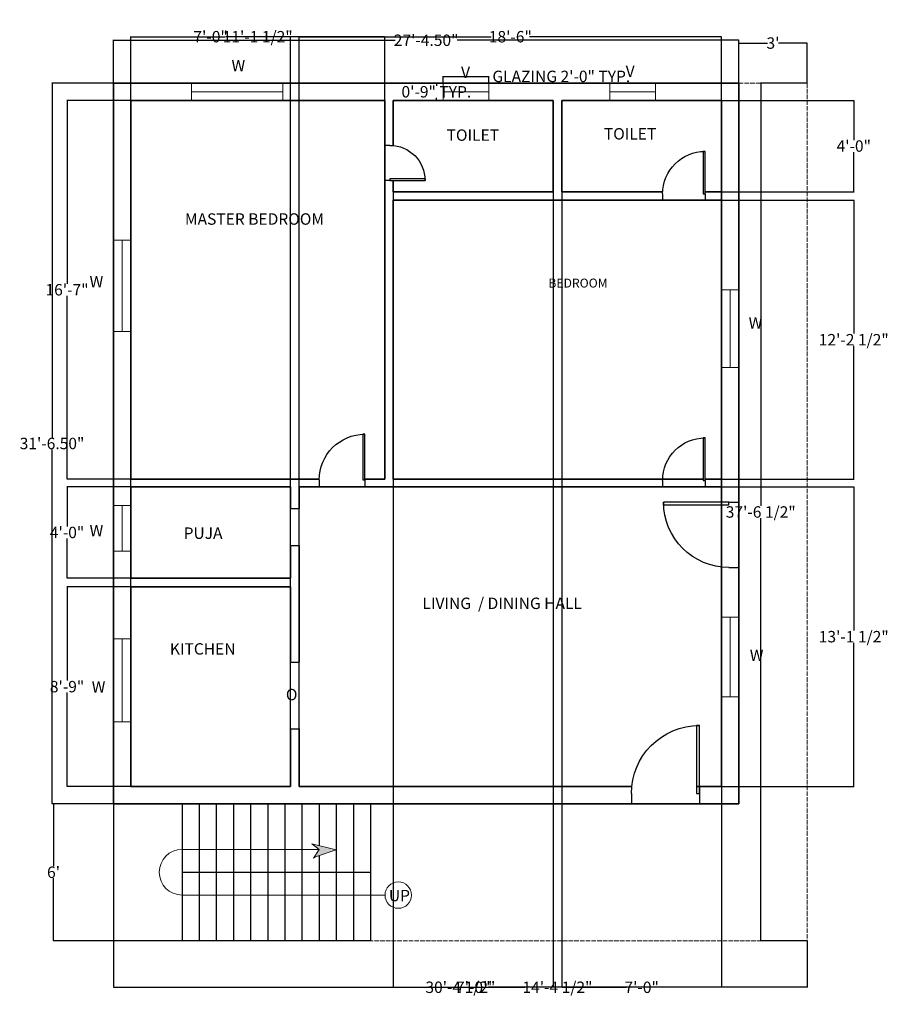
# Model space of a CAD drawing. Units: inches. Extents: x -21 to 896, y -151 to 366.
# Tile 2 of 2: x 440 to 896, y -151 to 366. Entities that reach past the tile are written whole.
import ezdxf

# ---------------------------------------------------------------- set-up
doc = ezdxf.new("R2010")
doc.units = ezdxf.units.IN
doc.header["$MEASUREMENT"] = 0
doc.linetypes.add('ACAD_ISO02W100', pattern=[15, 12, -3])
for name, color, linetype, lineweight in [('A-ANNO-DIMS', 2, 'Continuous', 18), ('A-ANNO-SYMB', 7, 'Continuous', 18), ('A-ANNO-TEXT', 7, 'Continuous', 18), ('A-AREA-IDEN', 7, 'Continuous', 25), ('A-DOOR', 3, 'Continuous', 25), ('A-FLOR-STRS', 7, 'Continuous', 25), ('A-GLAZ', 4, 'Continuous', 18), ('A-WALL', 7, 'Continuous', 35), ('A-WALL-OPEN', 7, 'ACAD_ISO02W100', 25), ('C-PROP', 8, 'ACAD_ISO02W100', 18)]:
    doc.layers.add(name, color=color, linetype=linetype, lineweight=lineweight)
doc.styles.get("Standard").update_dxf_attribs({"font": 'arial.ttf'})
doc.dimstyles.get("Standard").update_dxf_attribs({"dimtxt": 6, "dimasz": 0.18, "dimexe": 0.18, "dimexo": 0.0625, "dimgap": 0.09, "dimtad": 0, "dimtih": 1, "dimtoh": 1, "dimzin": 0, "dimdsep": 46, "dimlunit": 3, "dimtxsty": 'Standard', "dimcen": 0.09, "dimadec": 0, "dimazin": 0, "dimtfac": 1, "dimtofl": 0, "dimtmove": 0, "dimatfit": 3, "dimfxl": 1, "dimtolj": 1, "dimtzin": 0, "dimarcsym": 0})

# ---------------------------------------------------------------- blocks, each defined once
blk = doc.blocks.new('*U2')
for p, q in [((0, 0), (0, -6)), ((40, 0), (40, -6))]:
    blk.add_line(p, q)
blk.add_lwpolyline([(0, 0), (0, 40), (1.75, 40), (1.75, 0)], close=True)
blk.add_arc((0, 0), 40, 0, 90)
blk = doc.blocks.new('*D17')
at = {"layer": 'A-ANNO-DIMS', "color": 0, "lineweight": -2, "ltscale": 0.4, "transparency": 16777216}
for p, q in [((489.19, 332.75), (489.19, 355.46)), ((489.37, 355.28), (637.17, 355.28)), ((817.51, 355.28), (669.71, 355.28)), ((817.69, 332.75), (817.69, 355.46))]:
    blk.add_line(p, q, dxfattribs=at)
at = {"layer": 'A-ANNO-DIMS', "color": 0, "ltscale": 0.4, "transparency": 16777216}
for points in [[(489.37, 355.31), (489.37, 355.25), (489.19, 355.28)], [(817.51, 355.31), (817.51, 355.25), (817.69, 355.28)]]:
    blk.add_solid(points, dxfattribs=at)
at = {"layer": 'Defpoints', "color": 0, "ltscale": 0.4, "transparency": 16777216}
for p in [(817.69, 355.28), (489.19, 332.69), (817.69, 332.69)]:
    blk.add_point(p, dxfattribs=at)
at = {"layer": 'A-ANNO-DIMS', "color": 0, "ltscale": 0.4, "transparency": 16777216, "insert": (653.44, 355.28), "char_height": 6, "attachment_point": 5}
blk.add_mtext('\\A1;27\'-4.50"', dxfattribs=at)
blk = doc.blocks.new('*D18')
at = {"layer": 'A-ANNO-DIMS', "color": 0, "lineweight": -2, "ltscale": 0.4, "transparency": 16777216}
for p, q in [((489.13, 332.69), (456.69, 332.69)), ((456.87, 332.51), (456.87, 146.59)), ((456.87, -45.63), (456.87, 140.28)), ((489.13, -45.81), (456.69, -45.81))]:
    blk.add_line(p, q, dxfattribs=at)
at = {"layer": 'A-ANNO-DIMS', "color": 0, "ltscale": 0.4, "transparency": 16777216}
for points in [[(456.84, 332.51), (456.9, 332.51), (456.87, 332.69)], [(456.84, -45.63), (456.9, -45.63), (456.87, -45.81)]]:
    blk.add_solid(points, dxfattribs=at)
at = {"layer": 'Defpoints', "color": 0, "ltscale": 0.4, "transparency": 16777216}
for p in [(489.19, 332.69), (456.87, -45.81), (489.19, -45.81)]:
    blk.add_point(p, dxfattribs=at)
at = {"layer": 'A-ANNO-DIMS', "color": 0, "ltscale": 0.4, "transparency": 16777216, "insert": (456.87, 143.44), "char_height": 6, "attachment_point": 5}
blk.add_mtext('\\A1;31\'-6.50"', dxfattribs=at)
blk = doc.blocks.new('*D19')
at = {"layer": 'A-ANNO-DIMS', "color": 0, "lineweight": -2, "ltscale": 0.4, "transparency": 16777216}
for p, q in [((489.13, -45.81), (457.48, -45.81)), ((457.66, -45.99), (457.66, -78.66)), ((457.66, -117.63), (457.66, -84.97)), ((489.13, -117.81), (457.48, -117.81))]:
    blk.add_line(p, q, dxfattribs=at)
at = {"layer": 'A-ANNO-DIMS', "color": 0, "ltscale": 0.4, "transparency": 16777216}
for points in [[(457.63, -45.99), (457.69, -45.99), (457.66, -45.81)], [(457.63, -117.63), (457.69, -117.63), (457.66, -117.81)]]:
    blk.add_solid(points, dxfattribs=at)
at = {"layer": 'Defpoints', "color": 0, "ltscale": 0.4, "transparency": 16777216}
for p in [(489.19, -45.81), (457.66, -117.81), (489.19, -117.81)]:
    blk.add_point(p, dxfattribs=at)
at = {"layer": 'A-ANNO-DIMS', "color": 0, "ltscale": 0.4, "transparency": 16777216, "insert": (457.66, -81.81), "char_height": 6, "attachment_point": 5}
blk.add_mtext("\\A1;6'", dxfattribs=at)
blk = doc.blocks.new('*D20')
at = {"layer": 'A-ANNO-DIMS', "color": 0, "lineweight": -2, "ltscale": 0.4, "transparency": 16777216}
for p, q in [((817.69, 332.75), (817.69, 353.98)), ((817.87, 353.8), (832.84, 353.8)), ((853.51, 353.8), (838.54, 353.8)), ((853.69, 332.75), (853.69, 353.98))]:
    blk.add_line(p, q, dxfattribs=at)
at = {"layer": 'A-ANNO-DIMS', "color": 0, "ltscale": 0.4, "transparency": 16777216}
for points in [[(817.87, 353.83), (817.87, 353.77), (817.69, 353.8)], [(853.51, 353.83), (853.51, 353.77), (853.69, 353.8)]]:
    blk.add_solid(points, dxfattribs=at)
at = {"layer": 'Defpoints', "color": 0, "ltscale": 0.4, "transparency": 16777216}
for p in [(853.69, 353.8), (817.69, 332.69), (853.69, 332.69)]:
    blk.add_point(p, dxfattribs=at)
at = {"layer": 'A-ANNO-DIMS', "color": 0, "ltscale": 0.4, "transparency": 16777216, "insert": (835.69, 353.8), "char_height": 6, "attachment_point": 5}
blk.add_mtext("\\A1;3'", dxfattribs=at)
blk = doc.blocks.new('STAIR-RETURN-72IN')
for p, q in [((0, 72), (0, 0)), ((36, 72), (36, 0)), ((45, 72), (45, 0)), ((54, 72), (54, 0)), ((63, 72), (63, 0)), ((72, 72), (72, 0)), ((81, 72), (81, 0)), ((90, 72), (90, 0)), ((99, 72), (99, 0)), ((108, 72), (108, 50.05)), ((117, 72), (117, 0)), ((126, 72), (126, 0)), ((135, 72), (135, 0)), ((108, 44.67), (108, 0)), ((36, 36), (135, 36))]:
    blk.add_line(p, q)
blk.add_lwpolyline([(135, 0), (0, 0)])
blk = doc.blocks.new('STAIR-TRAVEL-UP')
h = blk.add_hatch(color=256)
h.dxf.hatch_style = 1
h.paths.add_polyline_path([(-32.62, 23.79), (-45.42, 26.99), (-41.62, 24), (-44.5, 19.46), (-43.01, 20.19)])
for p, q in [((-41.62, 24), (-45.42, 26.99)), ((-45.42, 26.99), (-32.62, 23.79)), ((-113.62, 24), (-41.62, 24)), ((-44.5, 19.46), (-41.62, 24)), ((-32.62, 23.79), (-43.01, 20.19)), ((-43.01, 20.19), (-44.5, 19.46)), ((-113.62, 0), (-14.62, 0)), ((-14.62, 0), (-6.96, 0))]:
    blk.add_line(p, q)
blk.add_circle((0, 0), 6.96)
blk.add_arc((-113.62, 12), 12, 90, 270)
at = {"insert": (-4.95, 2.74), "char_height": 6, "attachment_point": 1}
blk.add_mtext_dynamic_manual_height_columns('UP', width=3.031, gutter_width=1, heights=[0.203], dxfattribs=at)
blk = doc.blocks.new('WIN-48IN')
at = {"ltscale": 0.4}
for p, q in [((0, 9), (0, 0)), ((48, 9), (48, 0)), ((0, 4.5), (48, 4.5))]:
    blk.add_line(p, q, dxfattribs=at)
blk = doc.blocks.new('GLAZ-24IN')
at = {"ltscale": 0.4}
for p, q in [((0, 9), (0, 0)), ((24, 9), (24, 0)), ((0, 4.5), (24, 4.5))]:
    blk.add_line(p, q, dxfattribs=at)
blk = doc.blocks.new('*D27')
at = {"layer": 'A-ANNO-DIMS', "color": 0, "lineweight": -2, "ltscale": 0.4, "transparency": 16777216}
for p, q in [((662.4, 332.75), (662.4, 336.47)), ((662.58, 336.29), (686.22, 336.29)), ((686.4, 332.75), (686.4, 336.47)), ((686.4, 336.29), (686.58, 336.29))]:
    blk.add_line(p, q, dxfattribs=at)
at = {"layer": 'A-ANNO-DIMS', "color": 0, "ltscale": 0.4, "transparency": 16777216}
for points in [[(662.58, 336.32), (662.58, 336.26), (662.4, 336.29)], [(686.22, 336.32), (686.22, 336.26), (686.4, 336.29)]]:
    blk.add_solid(points, dxfattribs=at)
at = {"layer": 'Defpoints', "color": 0, "ltscale": 0.4, "transparency": 16777216}
for p in [(686.4, 336.29), (662.4, 332.69), (686.4, 332.69)]:
    blk.add_point(p, dxfattribs=at)
at = {"layer": 'A-ANNO-DIMS', "color": 0, "ltscale": 0.4, "transparency": 16777216, "insert": (724.47, 336.29), "char_height": 6, "attachment_point": 5}
blk.add_mtext('\\A1;GLAZING 2\'-0" TYP.', dxfattribs=at)
blk = doc.blocks.new('*D28')
at = {"layer": 'A-ANNO-DIMS', "color": 0, "lineweight": -2, "ltscale": 0.4, "transparency": 16777216}
for p, q in [((662.33, 332.69), (658.62, 332.69)), ((658.8, 332.51), (658.8, 331.34)), ((662.33, 323.69), (658.62, 323.69)), ((658.8, 323.87), (658.8, 325.03))]:
    blk.add_line(p, q, dxfattribs=at)
at = {"layer": 'A-ANNO-DIMS', "color": 0, "ltscale": 0.4, "transparency": 16777216}
for points in [[(658.77, 332.51), (658.83, 332.51), (658.8, 332.69)], [(658.77, 323.87), (658.83, 323.87), (658.8, 323.69)]]:
    blk.add_solid(points, dxfattribs=at)
at = {"layer": 'Defpoints', "color": 0, "ltscale": 0.4, "transparency": 16777216}
for p in [(658.8, 332.69), (662.4, 332.69), (662.4, 323.69)]:
    blk.add_point(p, dxfattribs=at)
at = {"layer": 'A-ANNO-DIMS', "color": 0, "ltscale": 0.4, "transparency": 16777216, "insert": (658.8, 328.19), "char_height": 6, "attachment_point": 5}
blk.add_mtext('\\A1;0\'-9" TYP.', dxfattribs=at)
blk = doc.blocks.new('*D33')
at = {"layer": 'A-ANNO-DIMS', "color": 0, "lineweight": -2, "ltscale": 0.4, "transparency": 16777216}
for p, q in [((498.19, 323.75), (498.19, 357.31)), ((498.37, 357.13), (547.84, 357.13)), ((631.51, 357.13), (582.04, 357.13)), ((631.69, 323.75), (631.69, 357.31))]:
    blk.add_line(p, q, dxfattribs=at)
at = {"layer": 'A-ANNO-DIMS', "color": 0, "ltscale": 0.4, "transparency": 16777216}
for points in [[(498.37, 357.16), (498.37, 357.1), (498.19, 357.13)], [(631.51, 357.16), (631.51, 357.1), (631.69, 357.13)]]:
    blk.add_solid(points, dxfattribs=at)
at = {"layer": 'Defpoints', "color": 0, "ltscale": 0.4, "transparency": 16777216}
for p in [(631.69, 357.13), (498.19, 323.69), (631.69, 323.69)]:
    blk.add_point(p, dxfattribs=at)
at = {"layer": 'A-ANNO-DIMS', "color": 0, "ltscale": 0.4, "transparency": 16777216, "insert": (564.94, 357.13), "char_height": 6, "attachment_point": 5}
blk.add_mtext('\\A1;11\'-1 1/2"', dxfattribs=at)
blk = doc.blocks.new('*D34')
at = {"layer": 'A-ANNO-DIMS', "color": 0, "lineweight": -2, "ltscale": 0.4, "transparency": 16777216}
for p, q in [((498.13, 323.69), (464.57, 323.69)), ((464.75, 323.51), (464.75, 227.34)), ((464.75, 124.87), (464.75, 221.03)), ((498.13, 124.69), (464.57, 124.69))]:
    blk.add_line(p, q, dxfattribs=at)
at = {"layer": 'A-ANNO-DIMS', "color": 0, "ltscale": 0.4, "transparency": 16777216}
for points in [[(464.72, 323.51), (464.78, 323.51), (464.75, 323.69)], [(464.72, 124.87), (464.78, 124.87), (464.75, 124.69)]]:
    blk.add_solid(points, dxfattribs=at)
at = {"layer": 'Defpoints', "color": 0, "ltscale": 0.4, "transparency": 16777216}
for p in [(464.75, 323.69), (498.19, 323.69), (498.19, 124.69)]:
    blk.add_point(p, dxfattribs=at)
at = {"layer": 'A-ANNO-DIMS', "color": 0, "ltscale": 0.4, "transparency": 16777216, "insert": (464.75, 224.19), "char_height": 6, "attachment_point": 5}
blk.add_mtext('\\A1;16\'-7"', dxfattribs=at)
blk = doc.blocks.new('*D35')
at = {"layer": 'A-ANNO-DIMS', "color": 0, "lineweight": -2, "ltscale": 0.4, "transparency": 16777216}
for p, q in [((636.19, 124.62), (636.19, -142.43)), ((808.69, 124.62), (808.69, -142.43)), ((636.37, -142.25), (705.34, -142.25)), ((808.51, -142.25), (739.54, -142.25))]:
    blk.add_line(p, q, dxfattribs=at)
at = {"layer": 'A-ANNO-DIMS', "color": 0, "ltscale": 0.4, "transparency": 16777216}
for points in [[(636.37, -142.22), (636.37, -142.28), (636.19, -142.25)], [(808.51, -142.22), (808.51, -142.28), (808.69, -142.25)]]:
    blk.add_solid(points, dxfattribs=at)
at = {"layer": 'Defpoints', "color": 0, "ltscale": 0.4, "transparency": 16777216}
for p in [(636.19, 124.69), (808.69, 124.69), (808.69, -142.25)]:
    blk.add_point(p, dxfattribs=at)
at = {"layer": 'A-ANNO-DIMS', "color": 0, "ltscale": 0.4, "transparency": 16777216, "insert": (722.44, -142.25), "char_height": 6, "attachment_point": 5}
blk.add_mtext('\\A1;14\'-4 1/2"', dxfattribs=at)
blk = doc.blocks.new('*D36')
at = {"layer": 'A-ANNO-DIMS', "color": 0, "lineweight": -2, "ltscale": 0.4, "transparency": 16777216}
for p, q in [((636.19, 275.62), (636.19, -142.43)), ((720.19, 275.62), (720.19, -142.43)), ((636.37, -142.25), (670.15, -142.25)), ((720.01, -142.25), (686.23, -142.25))]:
    blk.add_line(p, q, dxfattribs=at)
at = {"layer": 'A-ANNO-DIMS', "color": 0, "ltscale": 0.4, "transparency": 16777216}
for points in [[(636.37, -142.22), (636.37, -142.28), (636.19, -142.25)], [(720.01, -142.22), (720.01, -142.28), (720.19, -142.25)]]:
    blk.add_solid(points, dxfattribs=at)
at = {"layer": 'Defpoints', "color": 0, "ltscale": 0.4, "transparency": 16777216}
for p in [(636.19, 275.69), (720.19, 275.69), (720.19, -142.25)]:
    blk.add_point(p, dxfattribs=at)
at = {"layer": 'A-ANNO-DIMS', "color": 0, "ltscale": 0.4, "transparency": 16777216, "insert": (678.19, -142.25), "char_height": 6, "attachment_point": 5}
blk.add_mtext('\\A1;7\'-0"', dxfattribs=at)
blk = doc.blocks.new('*D37')
at = {"layer": 'A-ANNO-DIMS', "color": 0, "lineweight": -2, "ltscale": 0.4, "transparency": 16777216}
for p, q in [((724.69, 275.62), (724.69, -142.43)), ((808.69, 275.62), (808.69, -142.43)), ((724.87, -142.25), (758.65, -142.25)), ((808.51, -142.25), (774.73, -142.25))]:
    blk.add_line(p, q, dxfattribs=at)
at = {"layer": 'A-ANNO-DIMS', "color": 0, "ltscale": 0.4, "transparency": 16777216}
for points in [[(724.87, -142.22), (724.87, -142.28), (724.69, -142.25)], [(808.51, -142.22), (808.51, -142.28), (808.69, -142.25)]]:
    blk.add_solid(points, dxfattribs=at)
at = {"layer": 'Defpoints', "color": 0, "ltscale": 0.4, "transparency": 16777216}
for p in [(724.69, 275.69), (808.69, 275.69), (808.69, -142.25)]:
    blk.add_point(p, dxfattribs=at)
at = {"layer": 'A-ANNO-DIMS', "color": 0, "ltscale": 0.4, "transparency": 16777216, "insert": (766.69, -142.25), "char_height": 6, "attachment_point": 5}
blk.add_mtext('\\A1;7\'-0"', dxfattribs=at)
blk = doc.blocks.new('*D38')
at = {"layer": 'A-ANNO-DIMS', "color": 0, "lineweight": -2, "ltscale": 0.4, "transparency": 16777216}
for p, q in [((808.75, 323.69), (878.31, 323.69)), ((878.13, 323.51), (878.13, 302.84)), ((878.13, 275.87), (878.13, 296.53)), ((808.75, 275.69), (878.31, 275.69))]:
    blk.add_line(p, q, dxfattribs=at)
at = {"layer": 'A-ANNO-DIMS', "color": 0, "ltscale": 0.4, "transparency": 16777216}
for points in [[(878.1, 323.51), (878.16, 323.51), (878.13, 323.69)], [(878.1, 275.87), (878.16, 275.87), (878.13, 275.69)]]:
    blk.add_solid(points, dxfattribs=at)
at = {"layer": 'Defpoints', "color": 0, "ltscale": 0.4, "transparency": 16777216}
for p in [(808.69, 323.69), (878.13, 323.69), (808.69, 275.69)]:
    blk.add_point(p, dxfattribs=at)
at = {"layer": 'A-ANNO-DIMS', "color": 0, "ltscale": 0.4, "transparency": 16777216, "insert": (878.13, 299.69), "char_height": 6, "attachment_point": 5}
blk.add_mtext('\\A1;4\'-0"', dxfattribs=at)
blk = doc.blocks.new('*D39')
at = {"layer": 'A-ANNO-DIMS', "color": 0, "lineweight": -2, "ltscale": 0.4, "transparency": 16777216}
for p, q in [((808.75, 271.19), (878.31, 271.19)), ((878.13, 271.01), (878.13, 201.13)), ((878.13, 124.87), (878.13, 194.74)), ((808.75, 124.69), (878.31, 124.69))]:
    blk.add_line(p, q, dxfattribs=at)
at = {"layer": 'A-ANNO-DIMS', "color": 0, "ltscale": 0.4, "transparency": 16777216}
for points in [[(878.1, 271.01), (878.16, 271.01), (878.13, 271.19)], [(878.1, 124.87), (878.16, 124.87), (878.13, 124.69)]]:
    blk.add_solid(points, dxfattribs=at)
at = {"layer": 'Defpoints', "color": 0, "ltscale": 0.4, "transparency": 16777216}
for p in [(808.69, 271.19), (878.13, 271.19), (808.69, 124.69)]:
    blk.add_point(p, dxfattribs=at)
at = {"layer": 'A-ANNO-DIMS', "color": 0, "ltscale": 0.4, "transparency": 16777216, "insert": (878.13, 197.94), "char_height": 6, "attachment_point": 5}
blk.add_mtext('\\A1;12\'-2 1/2"', dxfattribs=at)
blk = doc.blocks.new('*D40')
at = {"layer": 'A-ANNO-DIMS', "color": 0, "lineweight": -2, "ltscale": 0.4, "transparency": 16777216}
for p, q in [((808.75, 120.69), (878.31, 120.69)), ((878.13, 120.51), (878.13, 45.13)), ((878.13, -36.63), (878.13, 38.74)), ((808.75, -36.81), (878.31, -36.81))]:
    blk.add_line(p, q, dxfattribs=at)
at = {"layer": 'A-ANNO-DIMS', "color": 0, "ltscale": 0.4, "transparency": 16777216}
for points in [[(878.1, 120.51), (878.16, 120.51), (878.13, 120.69)], [(878.1, -36.63), (878.16, -36.63), (878.13, -36.81)]]:
    blk.add_solid(points, dxfattribs=at)
at = {"layer": 'Defpoints', "color": 0, "ltscale": 0.4, "transparency": 16777216}
for p in [(808.69, 120.69), (878.13, 120.69), (808.69, -36.81)]:
    blk.add_point(p, dxfattribs=at)
at = {"layer": 'A-ANNO-DIMS', "color": 0, "ltscale": 0.4, "transparency": 16777216, "insert": (878.13, 41.94), "char_height": 6, "attachment_point": 5}
blk.add_mtext('\\A1;13\'-1 1/2"', dxfattribs=at)
blk = doc.blocks.new('*D41')
at = {"layer": 'A-ANNO-DIMS', "color": 0, "lineweight": -2, "ltscale": 0.4, "transparency": 16777216}
for p, q in [((498.19, -36.75), (498.19, 357.31)), ((498.37, 357.13), (532.15, 357.13)), ((582.01, 357.13), (548.23, 357.13)), ((582.19, -36.75), (582.19, 357.31))]:
    blk.add_line(p, q, dxfattribs=at)
at = {"layer": 'A-ANNO-DIMS', "color": 0, "ltscale": 0.4, "transparency": 16777216}
for points in [[(498.37, 357.16), (498.37, 357.1), (498.19, 357.13)], [(582.01, 357.16), (582.01, 357.1), (582.19, 357.13)]]:
    blk.add_solid(points, dxfattribs=at)
at = {"layer": 'Defpoints', "color": 0, "ltscale": 0.4, "transparency": 16777216}
for p in [(582.19, 357.13), (498.19, -36.81), (582.19, -36.81)]:
    blk.add_point(p, dxfattribs=at)
at = {"layer": 'A-ANNO-DIMS', "color": 0, "ltscale": 0.4, "transparency": 16777216, "insert": (540.19, 357.13), "char_height": 6, "attachment_point": 5}
blk.add_mtext('\\A1;7\'-0"', dxfattribs=at)
blk = doc.blocks.new('*D42')
at = {"layer": 'A-ANNO-DIMS', "color": 0, "lineweight": -2, "ltscale": 0.4, "transparency": 16777216}
for p, q in [((586.69, -36.75), (586.69, 357.31)), ((586.87, 357.13), (687.58, 357.13)), ((808.51, 357.13), (707.8, 357.13)), ((808.69, -36.75), (808.69, 357.31))]:
    blk.add_line(p, q, dxfattribs=at)
at = {"layer": 'A-ANNO-DIMS', "color": 0, "ltscale": 0.4, "transparency": 16777216}
for points in [[(586.87, 357.16), (586.87, 357.1), (586.69, 357.13)], [(808.51, 357.16), (808.51, 357.1), (808.69, 357.13)]]:
    blk.add_solid(points, dxfattribs=at)
at = {"layer": 'Defpoints', "color": 0, "ltscale": 0.4, "transparency": 16777216}
for p in [(808.69, 357.13), (586.69, -36.81), (808.69, -36.81)]:
    blk.add_point(p, dxfattribs=at)
at = {"layer": 'A-ANNO-DIMS', "color": 0, "ltscale": 0.4, "transparency": 16777216, "insert": (697.69, 357.13), "char_height": 6, "attachment_point": 5}
blk.add_mtext('\\A1;18\'-6"', dxfattribs=at)
blk = doc.blocks.new('*D43')
at = {"layer": 'A-ANNO-DIMS', "color": 0, "lineweight": -2, "ltscale": 0.4, "transparency": 16777216}
for p, q in [((498.13, 68.19), (464.57, 68.19)), ((464.75, 68.01), (464.75, 18.84)), ((464.75, -36.63), (464.75, 12.53)), ((498.13, -36.81), (464.57, -36.81))]:
    blk.add_line(p, q, dxfattribs=at)
at = {"layer": 'A-ANNO-DIMS', "color": 0, "ltscale": 0.4, "transparency": 16777216}
for points in [[(464.72, 68.01), (464.78, 68.01), (464.75, 68.19)], [(464.72, -36.63), (464.78, -36.63), (464.75, -36.81)]]:
    blk.add_solid(points, dxfattribs=at)
at = {"layer": 'Defpoints', "color": 0, "ltscale": 0.4, "transparency": 16777216}
for p in [(464.75, 68.19), (498.19, 68.19), (498.19, -36.81)]:
    blk.add_point(p, dxfattribs=at)
at = {"layer": 'A-ANNO-DIMS', "color": 0, "ltscale": 0.4, "transparency": 16777216, "insert": (464.75, 15.69), "char_height": 6, "attachment_point": 5}
blk.add_mtext('\\A1;8\'-9"', dxfattribs=at)
blk = doc.blocks.new('*D44')
at = {"layer": 'A-ANNO-DIMS', "color": 0, "lineweight": -2, "ltscale": 0.4, "transparency": 16777216}
for p, q in [((498.13, 120.69), (464.57, 120.69)), ((464.75, 120.51), (464.75, 99.84)), ((464.75, 72.87), (464.75, 93.53)), ((498.13, 72.69), (464.57, 72.69))]:
    blk.add_line(p, q, dxfattribs=at)
at = {"layer": 'A-ANNO-DIMS', "color": 0, "ltscale": 0.4, "transparency": 16777216}
for points in [[(464.72, 120.51), (464.78, 120.51), (464.75, 120.69)], [(464.72, 72.87), (464.78, 72.87), (464.75, 72.69)]]:
    blk.add_solid(points, dxfattribs=at)
at = {"layer": 'Defpoints', "color": 0, "ltscale": 0.4, "transparency": 16777216}
for p in [(464.75, 120.69), (498.19, 120.69), (498.19, 72.69)]:
    blk.add_point(p, dxfattribs=at)
at = {"layer": 'A-ANNO-DIMS', "color": 0, "ltscale": 0.4, "transparency": 16777216, "insert": (464.75, 96.69), "char_height": 6, "attachment_point": 5}
blk.add_mtext('\\A1;4\'-0"', dxfattribs=at)
blk = doc.blocks.new('*D45')
at = {"layer": 'A-ANNO-DIMS', "color": 0, "lineweight": -2, "ltscale": 0.4, "transparency": 16777216}
for p, q in [((853.63, 332.69), (829.07, 332.69)), ((829.25, 332.51), (829.25, 110.63)), ((829.25, -117.63), (829.25, 104.24)), ((853.63, -117.81), (829.07, -117.81))]:
    blk.add_line(p, q, dxfattribs=at)
at = {"layer": 'A-ANNO-DIMS', "color": 0, "ltscale": 0.4, "transparency": 16777216}
for points in [[(829.22, 332.51), (829.28, 332.51), (829.25, 332.69)], [(829.22, -117.63), (829.28, -117.63), (829.25, -117.81)]]:
    blk.add_solid(points, dxfattribs=at)
at = {"layer": 'Defpoints', "color": 0, "ltscale": 0.4, "transparency": 16777216}
for p in [(829.25, 332.69), (853.69, 332.69), (853.69, -117.81)]:
    blk.add_point(p, dxfattribs=at)
at = {"layer": 'A-ANNO-DIMS', "color": 0, "ltscale": 0.4, "transparency": 16777216, "insert": (829.25, 107.44), "char_height": 6, "attachment_point": 5}
blk.add_mtext('\\A1;37\'-6 1/2"', dxfattribs=at)
blk = doc.blocks.new('*D46')
at = {"layer": 'A-ANNO-DIMS', "color": 0, "lineweight": -2, "ltscale": 0.4, "transparency": 16777216}
for p, q in [((489.19, -117.88), (489.19, -142.43)), ((853.69, -117.88), (853.69, -142.43)), ((489.37, -142.25), (654.05, -142.25)), ((853.51, -142.25), (688.82, -142.25))]:
    blk.add_line(p, q, dxfattribs=at)
at = {"layer": 'A-ANNO-DIMS', "color": 0, "ltscale": 0.4, "transparency": 16777216}
for points in [[(489.37, -142.22), (489.37, -142.28), (489.19, -142.25)], [(853.51, -142.22), (853.51, -142.28), (853.69, -142.25)]]:
    blk.add_solid(points, dxfattribs=at)
at = {"layer": 'Defpoints', "color": 0, "ltscale": 0.4, "transparency": 16777216}
for p in [(489.19, -117.81), (853.69, -117.81), (853.69, -142.25)]:
    blk.add_point(p, dxfattribs=at)
at = {"layer": 'A-ANNO-DIMS', "color": 0, "ltscale": 0.4, "transparency": 16777216, "insert": (671.44, -142.25), "char_height": 6, "attachment_point": 5}
blk.add_mtext('\\A1;30\'-4 1/2"', dxfattribs=at)

msp = doc.modelspace()

# ---------------------------------------------------------------- linework, layer by layer
at = {"layer": 'A-DOOR'}
msp.add_line((797.01, -36.815), (797.01, -45.815), dxfattribs=at)
at = {"layer": 'A-GLAZ', "ltscale": 0.4}
for p, q in [((749.973, 323.685), (749.973, 332.685)), ((773.973, 323.685), (773.973, 332.685)), ((749.973, 328.145), (773.973, 328.185)), ((808.689, 224.185), (817.689, 224.185)), ((813.189, 183.392), (813.189, 224.185)), ((808.689, 183.392), (817.689, 183.392)), ((808.689, 52.137), (817.689, 52.137)), ((813.189, 10.257), (813.189, 52.137)), ((489.189, 40.836), (498.189, 40.836)), ((493.689, -2.772), (493.689, 40.836)), ((808.689, 10.257), (817.689, 10.257)), ((489.189, -2.772), (498.189, -2.772))]:
    msp.add_line(p, q, dxfattribs=at)
at = {"layer": 'A-WALL'}
msp.add_lwpolyline([(489.189, 332.685), (817.689, 332.685), (817.689, -45.815), (489.189, -45.815)], close=True, dxfattribs=at)
for points in [[(498.189, 323.685), (631.689, 323.685)], [(498.189, 124.685), (498.189, 323.685)], [(631.689, 124.685), (631.689, 323.685)], [(636.189, 323.685), (636.189, 299.953)], [(636.189, 323.685), (720.189, 323.685)], [(720.189, 323.685), (720.189, 275.685)], [(724.689, 323.685), (724.689, 275.685)], [(724.689, 323.685), (808.689, 323.685)], [(808.689, 323.685), (808.689, 124.685)], [(636.189, 281.612), (636.189, 275.685)], [(636.189, 275.685), (720.189, 275.685)], [(724.689, 275.685), (777.724, 275.685)], [(800.066, 275.685), (808.689, 275.685)], [(636.189, 271.185), (808.689, 271.185)], [(636.189, 271.185), (636.189, 124.685)], [(724.689, 271.185), (808.689, 271.185)], [(498.189, 124.685), (597.248, 124.685)], [(621.257, 124.685), (631.689, 124.685)], [(636.189, 124.685), (799.087, 124.685)], [(800.066, 124.685), (808.689, 124.685)], [(498.189, 120.685), (582.189, 120.685)], [(498.189, 72.685), (498.189, 120.685)], [(582.189, 109.238), (582.189, 120.685)], [(586.689, 120.685), (808.689, 120.685)], [(586.689, 109.238), (586.689, 120.685)], [(808.689, 120.685), (808.689, 112.622)], [(582.189, 72.685), (582.189, 89.787)], [(586.689, 28.488), (586.689, 89.787)], [(808.689, 78.478), (808.689, -36.815)], [(498.189, 72.685), (582.189, 72.685)], [(498.189, -36.815), (498.189, 68.185)], [(498.189, 68.185), (582.189, 68.185)], [(582.189, 28.488), (582.189, 68.185)], [(582.189, -36.815), (582.189, -6.471)], [(586.689, -36.815), (586.689, -6.471)], [(582.189, -36.815), (498.189, -36.815)], [(761.466, -36.815), (586.689, -36.815)], [(808.689, -36.815), (795.447, -36.815)]]:
    msp.add_lwpolyline(points, dxfattribs=at)
at = {"layer": 'A-WALL-OPEN', "ltscale": 0.4}
for p, q in [((582.189, 109.238), (586.689, 109.238)), ((582.189, 89.787), (586.689, 89.787)), ((582.189, 28.488), (586.689, 28.488)), ((582.189, -6.471), (586.689, -6.471))]:
    msp.add_line(p, q, dxfattribs=at)
at = {"layer": 'C-PROP', "ltscale": 0.2}
msp.add_line((817.689, 332.685), (853.689, 332.685), dxfattribs=at)
for points in [[(853.689, 332.685), (853.689, -117.815)], [(853.689, -117.815), (624.189, -117.815)]]:
    msp.add_lwpolyline(points, dxfattribs=at)

# ---------------------------------------------------------------- block references
at = {"layer": 'A-ANNO-SYMB'}
msp.add_blockref('STAIR-TRAVEL-UP', (638.811, -93.815), dxfattribs=at)
at = {"layer": 'A-DOOR'}
for p, xscale, yscale, zscale, rotation in [((634.429, 281.612), -0.4606261510920194, 0.4606261510920194, 0.4606261510920194, 270), ((812.535, 112.622), -0.8590067270063272, 0.8590067270063272, 0.8590067270063272, 90)]:
    msp.add_blockref('*U2', p, dxfattribs=dict(at, xscale=xscale, yscale=yscale, zscale=zscale, rotation=rotation))
for p, xscale, yscale, zscale in [((800.066, 274.541), -0.5592774159886474, 0.5592774159886474, 0.5592774159886474), ((621.257, 124.287), -0.6002384071363702, 0.6002384071363702, 0.6002384071363702), ((800.066, 124.041), -0.5592774159886474, 0.5592774159886474, 0.5592774159886474), ((797.01, -40.455), -0.8932506770278118, 0.8932506770278118, 0.8932506770278118)]:
    msp.add_blockref('*U2', p, dxfattribs=dict(at, xscale=xscale, yscale=yscale, zscale=zscale))
at = {"layer": 'A-FLOR-STRS'}
msp.add_blockref('STAIR-RETURN-72IN', (489.189, -117.815), dxfattribs=at)
at = {"layer": 'A-GLAZ'}
for name, p in [('WIN-48IN', (530.078, 323.685)), ('GLAZ-24IN', (662.396, 323.685))]:
    msp.add_blockref(name, p, dxfattribs=at)
at = {"layer": 'A-GLAZ', "rotation": 270}
for name, p in [('WIN-48IN', (489.189, 250.261)), ('GLAZ-24IN', (489.189, 110.854))]:
    msp.add_blockref(name, p, dxfattribs=at)

# ---------------------------------------------------------------- texts
at = {"layer": 'A-ANNO-TEXT', "char_height": 6, "attachment_point": 1}
for s, insert in [('W', (551.178, 344.962)), ('V', (671.786, 341.404)), ('V', (758.297, 341.993)), ('W', (476.601, 231.392)), ('W', (822.897, 209.769)), ('W', (476.601, 100.668)), ('W', (823.509, 35.165)), ('W', (477.72, 18.546)), ('O', (579.745, 14.495))]:
    msp.add_mtext_dynamic_manual_height_columns(s, width=6, gutter_width=1, heights=[0.203], dxfattribs=dict(at, insert=insert))
at = {"layer": 'A-AREA-IDEN', "attachment_point": 1}
for s, width, gutter_width, insert, char_height in [('TOILET', 173.95707, 1, (664.206, 308.431), 6), ('TOILET', 173.95707, 1, (746.842, 309.125), 6), ('MASTER BEDROOM', 173.95707, 1, (526.703, 264.353), 6), ('BEDROOM ', 135.93882, 0.781, (717.676, 230.055), 4.6887), ('PUJA', 173.95707, 1, (526.002, 99.315), 6), ('LIVING  / DINING HALL', 173.95707, 1, (651.514, 62.458), 6), ('KITCHEN ', 173.95707, 1, (518.805, 38.518), 6)]:
    msp.add_mtext_dynamic_manual_height_columns(s, width=width, gutter_width=gutter_width, heights=[0], dxfattribs=dict(at, insert=insert, char_height=char_height))

# ---------------------------------------------------------------- dimensions: what is measured, and where the dimension line sits
at = {"layer": 'A-ANNO-DIMS', "ltscale": 0.4}
for base, p1, p2, override, picture, middle in [((631.689, 357.125), (498.189, 323.685), (631.689, 323.685), {"dimdec": 1, "dimlfac": 1, "dimrnd": 0, "dimzin": 1, "dimdsep": 46, "dimlunit": 4, "dimfrac": 2}, '*D33', (564.939, 357.125)), ((817.689, 355.284), (489.189, 332.685), (817.689, 332.685), {"dimclrd": 0, "dimclre": 0, "dimclrt": 0}, '*D17', (653.439, 355.284)), ((582.189, 357.125), (498.189, -36.815), (582.189, -36.815), {"dimdec": 1, "dimlfac": 1, "dimrnd": 0, "dimzin": 1, "dimdsep": 46, "dimlunit": 4, "dimfrac": 2}, '*D41', (540.189, 357.125)), ((808.689, 357.125), (586.689, -36.815), (808.689, -36.815), {"dimdec": 1, "dimlfac": 1, "dimrnd": 0, "dimzin": 1, "dimdsep": 46, "dimlunit": 4, "dimfrac": 2}, '*D42', (697.689, 357.125)), ((853.689, 353.799), (817.689, 332.685), (853.689, 332.685), {"dimclrd": 0, "dimclre": 0, "dimclrt": 0}, '*D20', (835.689, 353.799)), ((720.189, -142.255), (636.189, 275.685), (720.189, 275.685), {"dimdec": 1, "dimlfac": 1, "dimrnd": 0, "dimzin": 1, "dimdsep": 46, "dimlunit": 4, "dimfrac": 2}, '*D36', (678.189, -142.255)), ((808.689, -142.255), (724.689, 275.685), (808.689, 275.685), {"dimdec": 1, "dimlfac": 1, "dimrnd": 0, "dimzin": 1, "dimdsep": 46, "dimlunit": 4, "dimfrac": 2}, '*D37', (766.689, -142.255)), ((808.689, -142.255), (636.189, 124.685), (808.689, 124.685), {"dimdec": 1, "dimlfac": 1, "dimrnd": 0, "dimzin": 1, "dimdsep": 46, "dimlunit": 4, "dimfrac": 2}, '*D35', (722.439, -142.255)), ((853.689, -142.255), (489.189, -117.815), (853.689, -117.815), {"dimdec": 1, "dimlfac": 1, "dimrnd": 0, "dimzin": 1, "dimdsep": 46, "dimlunit": 4, "dimfrac": 2}, '*D46', (671.439, -142.255))]:
    dim = msp.add_linear_dim(base=base, p1=p1, p2=p2, dimstyle='Standard', override=override, dxfattribs=at)
    dim.commit()
    dim.dimension.update_dxf_attribs({"geometry": picture, "text_midpoint": middle})
dim = msp.add_linear_dim(base=(686.396, 336.285), p1=(662.396, 332.685), p2=(686.396, 332.685), text='GLAZING <> TYP.', dimstyle='Standard', override={"dimdec": 1, "dimlfac": 1, "dimrnd": 0, "dimzin": 1, "dimdsep": 46, "dimlunit": 4, "dimfrac": 2}, dxfattribs=at)
dim.commit()
dim.dimension.update_dxf_attribs({"geometry": '*D27', "text_midpoint": (724.465, 336.285)})
dim = msp.add_linear_dim(base=(658.796, 332.685), p1=(662.396, 323.685), p2=(662.396, 332.685), angle=90, text='<> TYP.', dimstyle='Standard', override={"dimdec": 1, "dimlfac": 1, "dimrnd": 0, "dimzin": 1, "dimdsep": 46, "dimlunit": 4, "dimfrac": 2}, dxfattribs=at)
dim.commit()
dim.dimension.update_dxf_attribs({"geometry": '*D28', "text_midpoint": (658.796, 328.185)})
for base, p1, p2, override, picture, middle in [((456.867, -45.815), (489.189, 332.685), (489.189, -45.815), {"dimclrd": 0, "dimclre": 0, "dimclrt": 0}, '*D18', (456.867, 143.435)), ((829.249, 332.685), (853.689, -117.815), (853.689, 332.685), {"dimdec": 1, "dimlfac": 1, "dimrnd": 0, "dimzin": 1, "dimdsep": 46, "dimlunit": 4, "dimfrac": 2}, '*D45', (829.249, 107.435)), ((464.749, 323.685), (498.189, 124.685), (498.189, 323.685), {"dimdec": 1, "dimlfac": 1, "dimrnd": 0, "dimzin": 1, "dimdsep": 46, "dimlunit": 4, "dimfrac": 2}, '*D34', (464.749, 224.185)), ((878.129, 323.685), (808.689, 275.685), (808.689, 323.685), {"dimdec": 1, "dimlfac": 1, "dimrnd": 0, "dimzin": 1, "dimdsep": 46, "dimlunit": 4, "dimfrac": 2}, '*D38', (878.129, 299.685)), ((878.129, 271.185), (808.689, 124.685), (808.689, 271.185), {"dimdec": 1, "dimlfac": 1, "dimrnd": 0, "dimzin": 1, "dimdsep": 46, "dimlunit": 4, "dimfrac": 2}, '*D39', (878.129, 197.935)), ((464.749, 120.685), (498.189, 72.685), (498.189, 120.685), {"dimdec": 1, "dimlfac": 1, "dimrnd": 0, "dimzin": 1, "dimdsep": 46, "dimlunit": 4, "dimfrac": 2}, '*D44', (464.749, 96.685)), ((878.129, 120.685), (808.689, -36.815), (808.689, 120.685), {"dimdec": 1, "dimlfac": 1, "dimrnd": 0, "dimzin": 1, "dimdsep": 46, "dimlunit": 4, "dimfrac": 2}, '*D40', (878.129, 41.935)), ((464.749, 68.185), (498.189, -36.815), (498.189, 68.185), {"dimdec": 1, "dimlfac": 1, "dimrnd": 0, "dimzin": 1, "dimdsep": 46, "dimlunit": 4, "dimfrac": 2}, '*D43', (464.749, 15.685)), ((457.659, -117.815), (489.189, -45.815), (489.189, -117.815), {"dimclrd": 0, "dimclre": 0, "dimclrt": 0}, '*D19', (457.659, -81.815))]:
    dim = msp.add_linear_dim(base=base, p1=p1, p2=p2, angle=90, dimstyle='Standard', override=override, dxfattribs=at)
    dim.commit()
    dim.dimension.update_dxf_attribs({"geometry": picture, "text_midpoint": middle})

doc.saveas('drawing.dxf')
